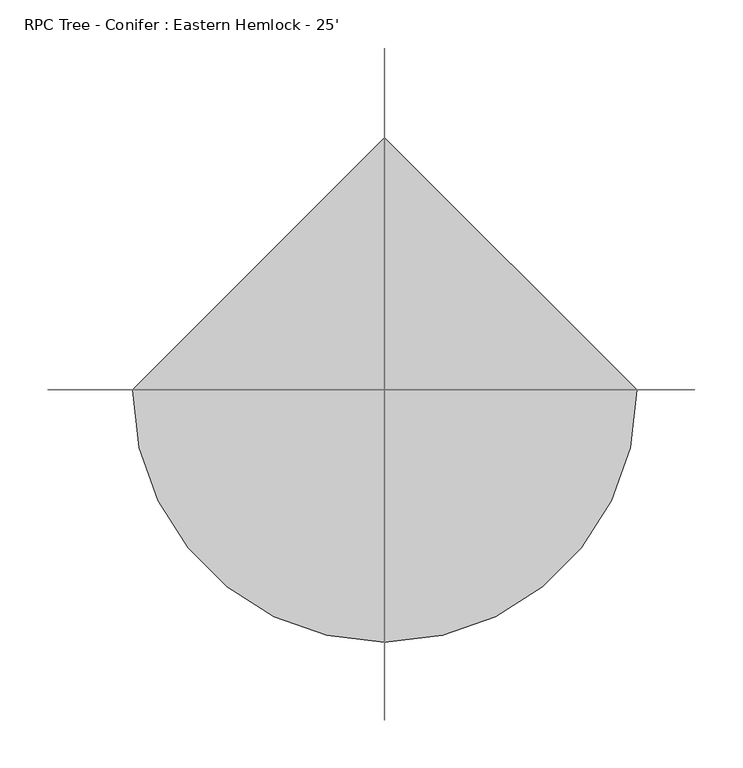
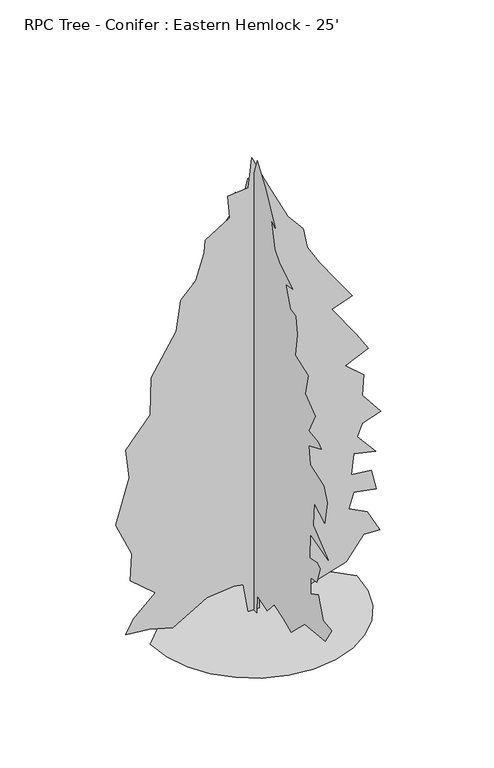
"""IFC4 building model written with IfcOpenShell, lengths in millimetres: geographic element geometry, RPC Tree - Conifer : Eastern Hemlock - 25'."""

from ifc_helpers import new_model, si_unit, origin, place, context, project, spatial, triangles, source, transform, mapped, element, save


def rpc_tree_conifer_eastern_hemlock_25_66632feb(model_context):
    return source(origin(), model_context, "Body", "Tessellation", [
        triangles([(-262.9954296, 0.0, 7.5e-06), (-256.0374604, -60.3060437, 7.5e-06), (-236.221428, -115.6877423, 7.5e-06), (-205.1338815, -164.558106, 7.5e-06), (-164.3614429, -205.3305446, 7.5e-06), (-115.4910701, -236.4180911, 7.5e-06), (-60.1093715, -256.2341236, 7.5e-06), (0.1966826, -263.1920928, 7.5e-06), (60.502716, -256.2341236, 7.5e-06), (115.8844146, -236.4180911, 7.5e-06), (164.7547691, -205.3305446, 7.5e-06), (205.5272078, -164.558106, 7.5e-06), (236.6147542, -115.6877423, 7.5e-06), (256.4307867, -60.3060437, 7.5e-06), (263.3887559, 2.3e-05, 7.5e-06), (0.1966366, 263.1920928, 7.5e-06), (-13.7718928, 6e-07, 1.2e-06), (-26.6734968, -3.4e-06, 77.4093648), (-50.3265202, -2.7e-06, 81.7098926), (-119.7659818, 8e-07, 74.6015556), (-206.1665401, 7.6e-06, 23.5182638), (-265.3525532, 9.2e-06, 40.8549463), (-325.5598157, 1.14e-05, 47.3057244), (-306.2074722, 8.5e-06, 81.7098926), (-250.3007285, 3e-06, 133.3161358), (-314.8085097, 2.5e-06, 189.2228977), (-310.5080091, -1.9e-06, 260.1819022), (-351.3629282, -5.5e-06, 350.4928142), (-316.9587782, -1.39e-05, 466.6077106), (-325.5598157, -1.82e-05, 544.0146137), (-263.2022847, -2.53e-05, 617.1259214), (-261.0520344, -3.13e-05, 716.0354364), (-196.5442168, -4.02e-05, 819.2487585), (-185.792929, -4.54e-05, 898.8095999), (-147.088233, -4.94e-05, 937.5150862), (-125.5856302, -5.45e-05, 1006.3225868), (-123.4353708, -5.65e-05, 1038.5785395), (-61.3070273, -6.16e-05, 1077.9871078), (-65.3783404, -6.49e-05, 1137.4880545), (-13.771852, -6.74e-05, 1141.787792), (-5.1710546, -7.24e-05, 1219.1987646), (29.2333923, -6.96e-05, 1146.0915264), (87.2905476, -6.52e-05, 1029.9750675), (125.9952255, -6.41e-05, 982.6701788), (136.7465314, -6.13e-05, 928.9116142), (166.8501718, -5.96e-05, 877.306988), (207.705109, -5.79e-05, 819.2487585), (250.7103147, -5.62e-05, 759.0406603), (199.1040715, -5.28e-05, 739.6919867), (261.4616206, -5.03e-05, 651.5276007), (291.5652519, -4.86e-05, 602.0728795), (233.5082397, -4.45e-05, 576.2705664), (280.8139641, -4.42e-05, 535.4152113), (276.5134453, -4.08e-05, 481.6607162), (323.8191879, -3.93e-05, 421.452618), (276.5134453, -3.63e-05, 406.3995761), (263.6118709, -3.38e-05, 374.1456945), (310.9176135, -3.26e-05, 318.2389326), (255.0108334, -3.09e-05, 331.1404707), (248.5600462, -2.74e-05, 277.3839772), (300.1663075, -2.93e-05, 270.93319), (313.067882, -2.66e-05, 217.1762787), (255.0108334, -2.47e-05, 227.9275846), (242.1092772, -2.17e-05, 187.0726474), (289.4150016, -2.24e-05, 163.4197852), (321.6689195, -2.02e-05, 103.2124954), (280.8139641, -1.85e-05, 105.3627548), (235.6584899, -1.31e-05, 47.3057244), (145.3475689, -7.5e-06, 19.3523412), (74.3889823, -5.9e-06, 45.1554651), (14.1814904, -5.4e-06, 79.5596332), (14.1814904, -6e-07, 0.0), (0.1966717, 14.6270119, 8.6e-06), (0.1966741, 25.3783542, 64.5078085), (0.1966763, 68.3836393, 73.1088506), (0.1966767, 87.7359783, 55.9067665), (0.1966797, 165.1453521, 40.8549463), (0.1966814, 212.4510766, 27.9534241), (0.1966844, 276.958876, 30.1036835), (0.1966876, 324.2646186, 68.8083273), (0.1966901, 356.5185001, 103.2124954), (0.1966875, 298.4614879, 103.2124954), (0.1966869, 253.3060138, 150.5182199), (0.1966901, 304.9122751, 180.6222599), (0.1966922, 339.3164251, 199.9746034), (0.196691, 285.5599317, 240.8295588), (0.1966938, 317.8138132, 285.9850147), (0.196693, 287.710182, 303.1871079), (0.196697, 326.414887, 378.4461951), (0.1966977, 328.5655552, 399.948807), (0.1966969, 302.7620067, 412.8491461), (0.1966981, 281.2594129, 485.9604538), (0.1967006, 298.4614879, 541.8647813), (0.196701, 287.710182, 571.9708652), (0.1967022, 276.958876, 627.8751926), (0.1967015, 229.6531516, 675.1841509), (0.1967044, 266.2075882, 718.1893747), (0.1967026, 201.6997706, 754.7409227), (0.196704, 208.1505578, 793.446409), (0.1967039, 173.7463896, 840.7513704), (0.1967057, 171.5961393, 905.2591335), (0.1967039, 126.0119123, 913.9033007), (0.1967056, 126.4406652, 967.6171005), (0.1967056, 79.1349408, 1038.5785395), (0.1967068, 81.2852001, 1075.1301601), (0.1967055, 46.8810365, 1083.7336321), (0.1967064, 25.3782724, 1146.0915264), (0.196706, -0.4248339, 1171.8938759), (0.1967067, -15.4766716, 1219.1987646), (0.1967034, -54.1815992, 1165.4402727), (0.1966992, -95.036541, 1085.8834282), (0.1967003, -77.834466, 1096.6326994), (0.1966976, -92.8862816, 1027.8251987), (0.196696, -112.2386251, 1004.1727907), (0.1966922, -172.4459058, 967.6171005), (0.1966934, -142.3422745, 963.3174356), (0.196691, -161.694618, 909.5629406), (0.1966897, -185.3474802, 903.1093374), (0.1966881, -191.7982492, 857.9542448), (0.1966866, -184.2912402, 796.8927103), (0.1966834, -241.2542421, 776.2435347), (0.1966823, -228.3526859, 720.3392435), (0.1966794, -271.3578916, 685.9334221), (0.196679, -243.4045106, 630.0250614), (0.196677, -284.2594478, 623.5754551), (0.1966761, -297.1610041, 612.8261839), (0.1966778, -243.4045106, 589.1737395), (0.1966761, -249.8552796, 541.8647813), (0.1966728, -310.0625785, 522.5120381), (0.196671, -325.114385, 485.9604538), (0.1966697, -314.3630791, 423.6024868), (0.1966725, -266.7956519, 448.2831388), (0.1966709, -262.7564362, 387.047269), (0.1966663, -329.414922, 333.2907392), (0.1966705, -249.8552796, 354.7933511), (0.1966687, -247.7050293, 290.2855335), (0.1966674, -279.9589291, 296.7363207), (0.1966666, -292.8604853, 288.1352832), (0.1966659, -277.8086606, 242.979809), (0.1966669, -252.0055481, 238.6792903), (0.1966656, -252.0055481, 195.6740846), (0.1966647, -284.2594478, 212.8761778), (0.196662, -307.91231, 156.968998), (0.1966602, -344.4667285, 152.6684793), (0.1966601, -316.5133475, 107.5130142), (0.1966639, -226.2024174, 98.9119676), (0.1966649, -165.9951367, 40.8549463), (0.1966668, -133.7412279, 55.9067665), (0.1966691, -90.7360223, 68.8083273), (0.1966694, -60.6323819, 34.4042045), (0.1966718, -15.4766307, 47.3057244), (0.1966705, -13.3263713, 7.7e-06)], [[15, 16, 1], [14, 15, 1], [14, 1, 2], [13, 14, 2], [13, 2, 3], [13, 3, 4], [12, 13, 4], [11, 12, 4], [11, 4, 5], [11, 5, 6], [11, 6, 7], [11, 7, 8], [11, 8, 9], [11, 9, 10], [40, 41, 42], [57, 58, 59], [65, 66, 67], [61, 62, 63], [60, 61, 63], [22, 23, 24], [54, 55, 56], [47, 48, 49], [50, 51, 52], [22, 24, 25], [71, 72, 17], [71, 17, 18], [38, 39, 40], [21, 22, 25], [20, 21, 25], [64, 65, 67], [40, 42, 43], [38, 40, 43], [64, 67, 68], [64, 68, 69], [64, 69, 70], [64, 70, 71], [49, 50, 52], [36, 37, 38], [36, 38, 43], [35, 36, 43], [35, 43, 44], [35, 44, 45], [35, 45, 46], [34, 35, 46], [33, 34, 46], [33, 46, 47], [33, 47, 49], [32, 33, 49], [31, 32, 49], [31, 49, 52], [30, 31, 52], [29, 30, 52], [28, 29, 52], [27, 28, 52], [27, 52, 53], [27, 53, 54], [27, 54, 56], [27, 56, 57], [27, 57, 59], [27, 59, 60], [26, 27, 60], [25, 26, 60], [20, 25, 60], [19, 20, 60], [18, 19, 60], [71, 18, 60], [64, 71, 60], [64, 60, 63], [133, 134, 135], [110, 111, 112], [114, 115, 116], [80, 81, 82], [108, 109, 110], [125, 126, 127], [124, 125, 127], [143, 144, 145], [84, 85, 86], [130, 131, 132], [96, 97, 98], [86, 87, 88], [141, 142, 143], [143, 145, 146], [141, 143, 146], [79, 80, 82], [151, 152, 73], [151, 73, 74], [120, 121, 122], [129, 130, 132], [128, 129, 132], [104, 105, 106], [122, 123, 124], [83, 84, 86], [100, 101, 102], [137, 138, 139], [136, 137, 139], [136, 139, 140], [78, 79, 82], [78, 82, 83], [77, 78, 83], [89, 90, 91], [146, 147, 148], [117, 118, 119], [149, 150, 151], [108, 110, 112], [107, 108, 112], [106, 107, 112], [106, 112, 113], [104, 106, 113], [76, 77, 83], [75, 76, 83], [88, 89, 91], [103, 104, 113], [102, 103, 113], [102, 113, 114], [102, 114, 116], [102, 116, 117], [102, 117, 119], [102, 119, 120], [100, 102, 120], [99, 100, 120], [98, 99, 120], [98, 120, 122], [98, 122, 124], [96, 98, 124], [96, 124, 127], [96, 127, 128], [96, 128, 132], [95, 96, 132], [94, 95, 132], [93, 94, 132], [92, 93, 132], [92, 132, 133], [92, 133, 135], [91, 92, 135], [88, 91, 135], [88, 135, 136], [86, 88, 136], [83, 86, 136], [75, 83, 136], [74, 75, 136], [74, 136, 140], [151, 74, 140], [149, 151, 140], [149, 140, 141], [149, 141, 146], [149, 146, 148]], closed=False),
    ])


if __name__ == "__main__":
    model = new_model("IFC4")
    model_context = context("Model", 3, world=origin())
    ifc_project = project(units=[si_unit("LENGTHUNIT", "METRE", prefix="MILLI")], contexts=[model_context])
    site = spatial("IfcSite", under=ifc_project)
    building = spatial("IfcBuilding", under=site)
    placement = place(None, origin())
    rpc_tree_conifer_eastern_hemlock_25_shape = rpc_tree_conifer_eastern_hemlock_25_66632feb(model_context)
    element("IfcGeographicElement", 1, ObjectType="RPC Tree - Conifer : Eastern Hemlock - 25'", at=placement, inside=building, context=model_context, shape_type="MappedRepresentation", body=[
        mapped(rpc_tree_conifer_eastern_hemlock_25_shape, transform((0.0, 0.0, 0.0), x_axis=(1.0, 0.0, 0.0), y_axis=(0.0, 1.0, 0.0), z_axis=(0.0, 0.0, 1.0))),
    ])
    save(model, "model.ifc")

# Revit data of these elements
# Type "RPC Tree - Conifer : Eastern Hemlock - 25'"
#   built-in parameter 1005198 = "{2, 15},{39, RPC-16-G0VH-QEXX-MT47-S000-ST1L-LVER-AU},{1, 0},{1, 0},{2, 13},{1, 8},{5, Color},{1, 0},{1, 0},{3, 0.8},{3, 0.8},{3, 0.8},{1, 8},{7, BBoxMin},{1, 0},{1, 0},{1, 0},{1, 0},{1, 0},{1, 8},{7, BBoxMax},{1, 0},{1, 0},{1, 0},{1, 0},{1, 0},{2, 11},{9, RPCTypeId},{1, 0},{1, 0},{39, RPC-16-G0VH-QEXX-MT47-S000-ST1L-LVER-AU},{1, 6},{14, RPCPlantHeight},{1, 0},{1, 0},{2, 25},{2, 11},{7, keyword},{1, 0},{1, 0},{34, :RPCs:Trees [General]:Geometry:RPC},{2, 11},{8, category},{1, 0},{1, 0},{15, Trees [General]},{2, 11},{12, LocalizedUID},{1, 0},{1, 0},{15, Eastern Hemlock},{2, 14},{6, Height},{1, 0},{1, 0},{2, 25},{1, 2},{16, Cast Reflections},{1, 0},{1, 0},{1, 0},{1, 2},{12, Cast Shadows},{1, 0},{1, 0},{1, 1},{1, 2},{9, Lock View},{1, 0},{1, 0},{1, 0},{1, 4},{5, ViewC},{1, 0},{1, 0},{1, 0},{21, assetlibrary_base.fbx},{1, 5},"
#   built-in parameter 1005195 = "RPC-16-G0VH-QEXX-MT47-S000-ST1L-LVER-AU"
#   Type Comments = "Eastern Hemlock"
#   Assembly Code = "G2050500"
#   Height = 4' - 0"
#   Description = (empty or 0)
#   Default Elevation = 0
